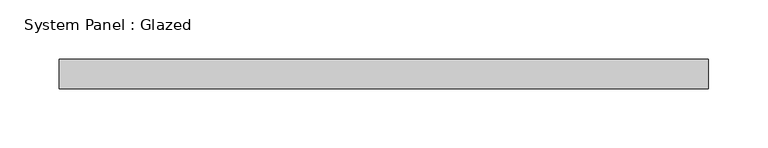
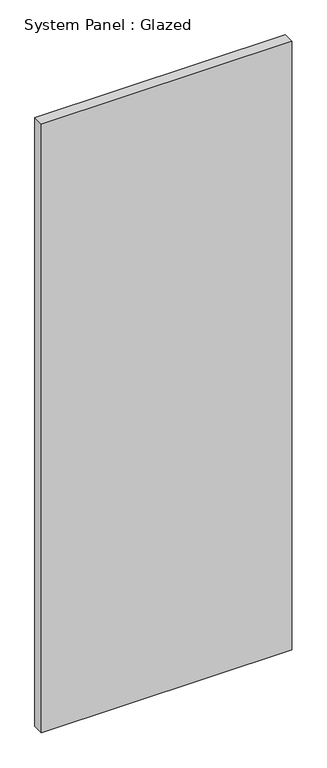
"""IFC4 building model written with IfcOpenShell, lengths in millimetres: plate geometry, System Panel : Glazed."""

from ifc_helpers import new_model, si_unit, origin, origin_with_axes, place, context, project, spatial, polyline, outline, extrude, source, transform, mapped, element, save


def system_panel_glazed_68fefaed(model_context):
    return source(origin(), model_context, "Body", "SweptSolid", [
        extrude(outline(polyline([(275.0, 24.5), (-275.0, 24.5), (-275.0, 49.5), (275.0, 49.5), (275.0, 24.5)])), origin_with_axes(), (0.0, 0.0, 1.0), 1415.0),
    ])


if __name__ == "__main__":
    model = new_model("IFC4")
    model_context = context("Model", 3, world=origin())
    ifc_project = project(units=[si_unit("LENGTHUNIT", "METRE", prefix="MILLI")], contexts=[model_context])
    site = spatial("IfcSite", under=ifc_project)
    building = spatial("IfcBuilding", under=site)
    placement = place(None, origin())
    system_panel_glazed_shape = system_panel_glazed_68fefaed(model_context)
    element("IfcPlate", 1, ObjectType="System Panel : Glazed", at=placement, inside=building, context=model_context, shape_type="MappedRepresentation", body=[
        mapped(system_panel_glazed_shape, transform((0.0, 0.0, 0.0), x_axis=(1.0, 0.0, 0.0), y_axis=(0.0, 1.0, 0.0), z_axis=(0.0, 0.0, 1.0))),
    ])
    save(model, "model.ifc")

# Revit data of these elements
# Type "System Panel : Glazed"
#   Construction Type Id = "GSP4R"
#   Analytic Construction = "1/8 in Pilkington single glazing"
#   Visual Light Transmittance = 0.9
#   Solar Heat Gain Coefficient = 0.86
#   Heat Transfer Coefficient (U) = 6.7069 W/(m²·K)
#   Define Thermal Properties by = 1
# Element 1 (IfcPlate, "System Panel : Glazed")
#   Materials on its faces: "Glass"
# Materials
#   "Glass": class "Glass", colour RGB 0 128 192, transparency 0.9, Description = "Soda Lime Glass", Cost = 0
